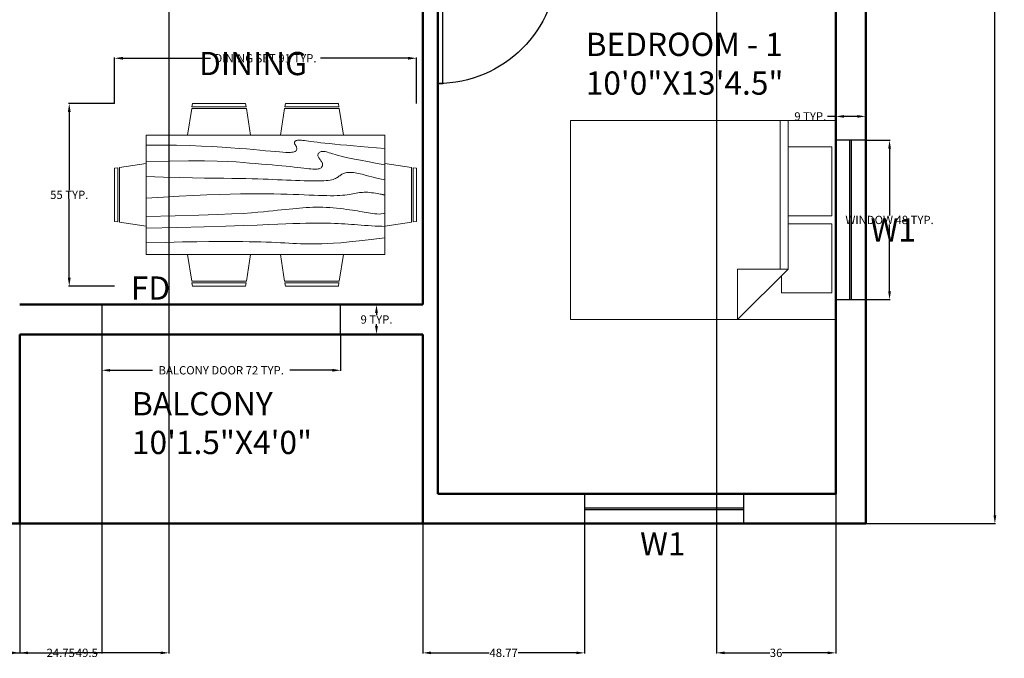
# Model space of a CAD drawing. Units: inches. Extents: x 227 to 711, y 218 to 1048.
# Tile 2 of 5: x 414 to 711, y 218 to 411. Entities that reach past the tile are written whole.
import ezdxf

# ---------------------------------------------------------------- set-up
doc = ezdxf.new("R2010")
doc.units = ezdxf.units.IN
doc.header["$MEASUREMENT"] = 0
for name, color, linetype, lineweight in [('A-ANNO-DIMS', 2, 'Continuous', 18), ('A-ANNO-TEXT', 70, 'Continuous', 18), ('A-AREA-IDEN', 70, 'Continuous', 25), ('A-FURN', 8, 'Continuous', 18), ('A-WALL', 10, 'Continuous', 50), ('DOORS', 30, 'Continuous', 25), ('WINDOWS', 50, 'Continuous', 25)]:
    doc.layers.add(name, color=color, linetype=linetype, lineweight=lineweight)
doc.styles.get("Standard").update_dxf_attribs({"font": 'arial.ttf'})
doc.dimstyles.get("Standard").update_dxf_attribs({"dimtxt": 2.5, "dimasz": 2.5, "dimexe": 0.18, "dimexo": 0.0625, "dimgap": 0.09, "dimtad": 0, "dimtih": 1, "dimtoh": 1, "dimzin": 0, "dimdsep": 46, "dimlunit": 3, "dimtxsty": 'Standard', "dimcen": 0.09, "dimadec": 0, "dimazin": 0, "dimtfac": 1, "dimtofl": 0, "dimtmove": 0, "dimatfit": 3, "dimfxl": 1, "dimtolj": 1, "dimtzin": 0, "dimarcsym": 0})

# ---------------------------------------------------------------- blocks, each defined once
blk = doc.blocks.new('*U2')
for p, q in [((0, 0), (0, -6)), ((40, 0), (40, -6))]:
    blk.add_line(p, q)
blk.add_lwpolyline([(0, 0), (0, 40), (1.75, 40), (1.75, 0)], close=True)
blk.add_arc((0, 0), 40, 0, 90)
blk = doc.blocks.new('Bed - Queen')
for p, q in [((0, -80.00003), (0, 0)), ((0, 0), (59.99999, 0)), ((59.99999, 0), (59.99999, -80.00003)), ((7.99999, -1.2), (28.79998, -1.2)), ((7.99999, -14.4), (7.99999, -1.2)), ((28.79998, -1.2), (28.79998, -14.4)), ((31.19999, -1.2), (51.99999, -1.2)), ((31.19999, -14.4), (31.19999, -1.2)), ((51.99999, -1.2), (51.99999, -16.4)), ((0, -14.4), (44.8, -14.4)), ((59.99999, -29.6), (44.8, -14.4)), ((44.8, -14.4), (44.8, -29.6)), ((44.8, -16.8), (0, -16.8)), ((51.99999, -16.4), (46.79936, -16.4)), ((44.8, -29.6), (59.99999, -29.6)), ((59.99999, -80.00003), (0, -80.00003))]:
    blk.add_line(p, q)
blk = doc.blocks.new('Dining Set - 36 x 72 in.')
for p, q in [((-22, 27.5), (-22.1562, 26.50042)), ((-22, 27.5), (-6, 27.5)), ((-5.8437, 26.49966), (-6, 27.5)), ((6, 27.5), (5.8438, 26.50042)), ((6, 27.5), (22, 27.5)), ((22.1563, 26.49966), (22, 27.5)), ((-22.2343, 26.00059), (-23.4847, 17.99762)), ((-22.2304, 26), (-5.7608, 26)), ((-5.8416, 26.5), (-22.1534, 26.5)), ((-4.5152, 17.99762), (-5.7655, 25.99926)), ((5.7657, 26.00059), (4.5153, 17.99762)), ((5.7696, 26), (22.2392, 26)), ((22.1584, 26.5), (5.8466, 26.5)), ((23.4848, 17.99762), (22.2345, 25.99926)), ((36, 18), (-36, 18)), ((-36, 18), (-36, -18)), ((36, -18), (36, 18)), ((-44.0006, 8.23428), (-35.9976, 9.48474)), ((44.0006, 8.23428), (35.9976, 9.48474)), ((-45.5, 8), (-44.5004, 8.15617)), ((-45.5, 8), (-45.5, -8)), ((-44.5, -8.15843), (-44.5, 8.15338)), ((-44, 8.23041), (-44, -8.23915)), ((44, 8.23041), (44, -8.23915)), ((44.5, -8.15843), (44.5, 8.15338)), ((45.5, 8), (44.5005, 8.15617)), ((45.5, 8), (45.5, -8)), ((-44.4997, -8.15631), (-45.5, -8)), ((-35.9976, -9.48476), (-43.9993, -8.2345)), ((35.9976, -9.48476), (43.9993, -8.2345)), ((44.4997, -8.15631), (45.5, -8)), ((-36, -18), (36, -18)), ((-22.2343, -26.0006), (-23.4847, -17.99762)), ((-4.5152, -17.99762), (-5.7655, -25.99928)), ((5.7657, -26.0006), (4.5153, -17.99762)), ((23.4848, -17.99762), (22.2345, -25.99928)), ((-22.2304, -26), (-5.7608, -26)), ((-22, -27.5), (-22.1562, -26.50044)), ((-5.8416, -26.5), (-22.1534, -26.5)), ((-5.8437, -26.49967), (-6, -27.5)), ((5.7696, -26), (22.2392, -26)), ((6, -27.5), (5.8438, -26.50044)), ((22.1584, -26.5), (5.8466, -26.5)), ((22.1563, -26.49967), (22, -27.5)), ((-22, -27.5), (-6, -27.5)), ((6, -27.5), (22, -27.5))]:
    blk.add_line(p, q)
for points in [[(-36, 15), (-31.1772, 14.97754), (-26.8079, 14.91406), (-22.8538, 14.81543), (-19.276, 14.6875), (-16.0362, 14.53613), (-13.0957, 14.36718), (-10.4159, 14.18652), (-7.9583, 14), (-5.6904, 13.81315), (-3.6035, 13.63021), (-1.6954, 13.45508), (0.0365, 13.29166), (1.5945, 13.14388), (2.9811, 13.01562), (4.1988, 12.9108), (5.25, 12.83333), (6.1393, 12.78613), (6.8802, 12.76823), (7.4883, 12.77767), (7.9792, 12.8125), (8.3685, 12.87077), (8.6719, 12.95052), (8.9049, 13.0498), (9.0833, 13.16666), (9.2205, 13.29899), (9.3216, 13.44401), (9.3895, 13.59879), (9.4271, 13.76041), (9.4373, 13.92594), (9.4232, 14.09245), (9.3875, 14.257), (9.3333, 14.41666), (9.2638, 14.56917), (9.1836, 14.71484), (9.0975, 14.85465), (9.0104, 14.98958), (8.9272, 15.1206), (8.8529, 15.2487), (8.7922, 15.37483), (8.75, 15.5), (8.7305, 15.62467), (8.7344, 15.74739), (8.7617, 15.86621), (8.8125, 15.97916), (8.8867, 16.08431), (8.9844, 16.17968), (9.1055, 16.26334), (9.25, 16.33333), (9.4189, 16.38802), (9.6172, 16.42708), (9.8506, 16.45052), (10.125, 16.45833), (10.4463, 16.45052), (10.8203, 16.42708), (11.2529, 16.38802), (11.75, 16.33333), (12.3184, 16.26318), (12.9694, 16.17838), (13.7151, 16.07991), (14.5677, 15.96875), (15.5395, 15.84586), (16.6426, 15.71224), (17.8893, 15.56884), (19.2917, 15.41666), (20.859, 15.25667), (22.5879, 15.08984), (24.4721, 14.91715), (26.5052, 14.73958), (28.6809, 14.5581), (30.9929, 14.3737), (33.4347, 14.18733), (36, 14)], [(-36, 10), (-28.9766, 10.14274), (-23.1725, 10.20442), (-18.4241, 10.19775), (-14.5677, 10.13541), (-11.4399, 10.03011), (-8.877, 9.89453), (-6.7154, 9.74137), (-4.7917, 9.58333), (-2.9698, 9.43082), (-1.2246, 9.28515), (0.4415, 9.14534), (2.026, 9.01041), (3.5266, 8.87939), (4.9408, 8.7513), (6.266, 8.62516), (7.5, 8.5), (8.6411, 8.37549), (9.6914, 8.2539), (10.6538, 8.13818), (11.5312, 8.03125), (12.3267, 7.93603), (13.043, 7.85547), (13.6831, 7.79248), (14.25, 7.75), (14.7471, 7.7303), (15.1797, 7.73307), (15.5537, 7.75732), (15.875, 7.80208), (16.1494, 7.86637), (16.3828, 7.94922), (16.5811, 8.04964), (16.75, 8.16666), (16.8944, 8.29915), (17.0143, 8.44531), (17.1089, 8.60319), (17.1771, 8.77083), (17.218, 8.94629), (17.2305, 9.1276), (17.2137, 9.31282), (17.1667, 9.5), (17.0895, 9.6875), (16.987, 9.875), (16.8649, 10.0625), (16.7292, 10.25), (16.5856, 10.4375), (16.4401, 10.625), (16.2985, 10.8125), (16.1667, 11), (16.05, 11.18733), (15.9518, 11.3737), (15.8752, 11.5581), (15.8229, 11.73958), (15.798, 11.91715), (15.8034, 12.08984), (15.842, 12.25667), (15.9167, 12.41666), (16.0295, 12.56836), (16.1784, 12.70833), (16.3605, 12.83268), (16.5729, 12.9375), (16.8127, 13.01888), (17.0768, 13.07291), (17.3625, 13.0957), (17.6667, 13.08333), (17.9894, 13.03312), (18.3418, 12.94726), (18.7382, 12.82918), (19.1927, 12.68229), (19.7195, 12.51001), (20.3327, 12.31575), (21.0465, 12.10294), (21.875, 11.875), (22.8357, 11.63354), (23.959, 11.37304), (25.2786, 11.08618), (26.8282, 10.76562), (28.6414, 10.40405), (30.752, 9.99414), (33.1936, 9.52856), (36, 9)], [(-36, 5.5), (-30.7157, 5.3348), (-26.069, 5.20963), (-21.9946, 5.11767), (-18.4271, 5.05208), (-15.3009, 5.00602), (-12.5508, 4.97265), (-10.1112, 4.94515), (-7.9167, 4.91666), (-5.909, 4.88167), (-4.0586, 4.83984), (-2.3429, 4.79215), (-0.7396, 4.73958), (0.7739, 4.6831), (2.22, 4.6237), (3.6213, 4.56233), (5, 4.5), (6.373, 4.43782), (7.7344, 4.3776), (9.0723, 4.32129), (10.375, 4.27083), (11.6309, 4.22819), (12.8281, 4.19531), (13.9551, 4.17415), (15, 4.16666), (15.954, 4.17448), (16.819, 4.19791), (17.6001, 4.23698), (18.3021, 4.29166), (18.9299, 4.36198), (19.4883, 4.44791), (19.9823, 4.54948), (20.4167, 4.66666), (20.7969, 4.79899), (21.1302, 4.94401), (21.4245, 5.09879), (21.6875, 5.26041), (21.9271, 5.42594), (22.1511, 5.59245), (22.3672, 5.757), (22.5834, 5.91666), (22.8065, 6.06868), (23.0404, 6.21093), (23.2879, 6.34147), (23.5521, 6.45833), (23.8358, 6.55957), (24.142, 6.64323), (24.4735, 6.70735), (24.8334, 6.75), (25.2235, 6.76969), (25.642, 6.76692), (26.0858, 6.74267), (26.5521, 6.69791), (27.0379, 6.63362), (27.5404, 6.55078), (28.0565, 6.45036), (28.5834, 6.33333), (29.1242, 6.19987), (29.7071, 6.04687), (30.3661, 5.87044), (31.1354, 5.66666), (32.0493, 5.43164), (33.142, 5.16146), (34.4475, 4.85221), (36, 4.5)], [(-36, -1), (-30.7915, -0.6591), (-26.0195, -0.38216), (-21.6519, -0.16284), (-17.6563, 0.00521), (-14.0005, 0.12833), (-10.6523, 0.21289), (-7.5796, 0.26522), (-4.75, 0.29166), (-2.134, 0.29793), (0.2878, 0.28711), (2.5317, 0.26163), (4.6146, 0.22396), (6.5529, 0.17651), (8.3633, 0.12174), (10.0623, 0.06209), (11.6667, 0), (13.1899, -0.06201), (14.6341, -0.1211), (15.9982, -0.17432), (17.2813, -0.21875), (18.4823, -0.25147), (19.6003, -0.26953), (20.6343, -0.27002), (21.5834, -0.25), (22.4481, -0.20768), (23.2357, -0.14584), (23.9549, -0.06836), (24.6146, 0.02083), (25.2235, 0.11784), (25.7904, 0.21875), (26.3241, 0.31966), (26.8334, 0.41666), (27.3265, 0.50618), (27.8099, 0.58593), (28.2894, 0.65397), (28.7709, 0.70833), (29.2601, 0.74707), (29.763, 0.76823), (30.2855, 0.76985), (30.8334, 0.75), (31.4088, 0.70784), (31.9994, 0.64713), (32.589, 0.57275), (33.1615, 0.48958), (33.7008, 0.4025), (34.1908, 0.3164), (34.6153, 0.23616), (34.9584, 0.16666), (35.2099, 0.11165), (35.3848, 0.07031), (35.504, 0.04069), (35.5886, 0.02083), (35.6594, 0.00879), (35.7377, 0.0026), (35.8442, 0.00032), (36, 0)], [(-36, -6.5), (-27.1843, -6.31267), (-20.084, -6.1263), (-14.469, -5.9419), (-10.1094, -5.76042), (-6.7752, -5.58285), (-4.2363, -5.41016), (-2.2629, -5.24333), (-0.625, -5.08334), (0.8708, -4.93099), (2.2715, -4.78646), (3.5872, -4.64974), (4.8281, -4.52084), (6.0046, -4.39974), (7.127, -4.28646), (8.2053, -4.18099), (9.25, -4.08334), (10.2705, -3.99382), (11.2734, -3.91407), (12.2647, -3.84603), (13.25, -3.79167), (14.2354, -3.75293), (15.2266, -3.73177), (16.2295, -3.73015), (17.25, -3.75), (18.2912, -3.79248), (19.3451, -3.85547), (20.4009, -3.93604), (21.4479, -4.03125), (22.4754, -4.13819), (23.4727, -4.25391), (24.4289, -4.37549), (25.3334, -4.5), (26.1785, -4.62492), (26.9694, -4.74935), (27.7145, -4.87281), (28.4219, -4.99479), (29.1, -5.11483), (29.7572, -5.23242), (30.4016, -5.34709), (31.0417, -5.45834), (31.6837, -5.56437), (32.3262, -5.65821), (32.9658, -5.73153), (33.599, -5.77604), (34.2224, -5.78345), (34.8327, -5.74545), (35.4264, -5.65373), (36, -5.5)], [(-36, -10), (-26.4022, -9.81299), (-18.4675, -9.62891), (-11.9839, -9.45069), (-6.7396, -9.28125), (-2.5226, -9.12354), (0.8789, -8.98047), (3.6769, -8.85498), (6.0833, -8.75), (8.2767, -8.66765), (10.3021, -8.60677), (12.1712, -8.56543), (13.8958, -8.54167), (15.4876, -8.53353), (16.9583, -8.53907), (18.3197, -8.55632), (19.5834, -8.58334), (20.7616, -8.61841), (21.8685, -8.66081), (22.9188, -8.71004), (23.9271, -8.76563), (24.9081, -8.82707), (25.8763, -8.89388), (26.8465, -8.96558), (27.8334, -9.04167), (28.8474, -9.12118), (29.8828, -9.20117), (30.93, -9.27824), (31.9792, -9.34896), (33.0205, -9.40991), (34.0443, -9.45768), (35.0407, -9.48885), (36, -9.5)], [(-36, -14.5), (-30.0881, -14.33513), (-25.0332, -14.21224), (-20.7312, -14.12647), (-17.0781, -14.07292), (-13.97, -14.04671), (-11.3027, -14.04297), (-8.9724, -14.05681), (-6.875, -14.08334), (-4.9224, -14.11833), (-3.0905, -14.16016), (-1.3709, -14.20785), (0.2448, -14.26042), (1.7647, -14.3169), (3.1973, -14.3763), (4.5507, -14.43767), (5.8333, -14.5), (7.0554, -14.5621), (8.235, -14.62175), (9.3922, -14.67652), (10.5469, -14.72396), (11.7192, -14.76164), (12.929, -14.78711), (14.1965, -14.79794), (15.5417, -14.79167), (16.9933, -14.76424), (18.6152, -14.70508), (20.4804, -14.60197), (22.6615, -14.44271), (25.2312, -14.21509), (28.2624, -13.9069), (31.8277, -13.50594), (36, -13)]]:
    blk.add_lwpolyline(points)
blk = doc.blocks.new('WIN-48IN')
for p, q in [((0, 4.75), (48, 4.75)), ((0, 4.25), (48, 4.25))]:
    blk.add_line(p, q)
blk.add_lwpolyline([(0, 0), (48, 0), (48, 9), (0, 9)], close=True)
blk = doc.blocks.new('DOOR-FD-72IN')
blk.add_lwpolyline([(0, 0), (72, 0), (72, 9), (0, 9)], close=True)
blk = doc.blocks.new('*D20')
at = {"layer": 'A-ANNO-DIMS', "color": 0, "lineweight": -2, "transparency": 16777216}
for p, q in [((669.55, 374.57), (676.87, 374.57)), ((676.69, 372.07), (676.69, 351.95)), ((676.69, 329.07), (676.69, 349.18)), ((669.55, 326.57), (676.87, 326.57))]:
    blk.add_line(p, q, dxfattribs=at)
at = {"layer": 'A-ANNO-DIMS', "color": 0, "transparency": 16777216}
for points in [[(676.27, 372.07), (677.11, 372.07), (676.69, 374.57)], [(676.27, 329.07), (677.11, 329.07), (676.69, 326.57)]]:
    blk.add_solid(points, dxfattribs=at)
at = {"layer": 'Defpoints', "color": 0, "transparency": 16777216}
for p in [(669.49, 374.57), (676.69, 374.57), (669.49, 326.57)]:
    blk.add_point(p, dxfattribs=at)
at = {"layer": 'A-ANNO-DIMS', "color": 0, "transparency": 16777216, "insert": (676.69, 350.57), "char_height": 2.5, "attachment_point": 5}
blk.add_mtext('\\A1;WINDOW 48 TYP.', dxfattribs=at)
blk = doc.blocks.new('*D21')
at = {"layer": 'A-ANNO-DIMS', "color": 0, "lineweight": -2, "transparency": 16777216}
for p, q in [((660.49, 381.77), (657.99, 381.77)), ((660.49, 374.63), (660.49, 381.95)), ((666.99, 381.77), (662.99, 381.77)), ((669.49, 374.63), (669.49, 381.95))]:
    blk.add_line(p, q, dxfattribs=at)
at = {"layer": 'A-ANNO-DIMS', "color": 0, "transparency": 16777216}
for points in [[(662.99, 382.18), (662.99, 381.35), (660.49, 381.77)], [(666.99, 382.18), (666.99, 381.35), (669.49, 381.77)]]:
    blk.add_solid(points, dxfattribs=at)
at = {"layer": 'Defpoints', "color": 0, "transparency": 16777216}
for p in [(660.49, 381.77), (660.49, 374.57), (669.49, 374.57)]:
    blk.add_point(p, dxfattribs=at)
at = {"layer": 'A-ANNO-DIMS', "color": 0, "transparency": 16777216, "insert": (652.79, 381.77), "char_height": 2.5, "attachment_point": 5}
blk.add_mtext('\\A1;9 TYP.', dxfattribs=at)
blk = doc.blocks.new('*D36')
at = {"layer": 'A-ANNO-DIMS', "color": 0, "lineweight": -2, "transparency": 16777216}
for p, q in [((443.08, 385.7), (443.08, 399.47)), ((445.58, 399.29), (471.99, 399.29)), ((531.58, 399.29), (505.17, 399.29)), ((534.08, 385.7), (534.08, 399.47))]:
    blk.add_line(p, q, dxfattribs=at)
at = {"layer": 'A-ANNO-DIMS', "color": 0, "transparency": 16777216}
for points in [[(445.58, 399.71), (445.58, 398.87), (443.08, 399.29)], [(531.58, 399.71), (531.58, 398.87), (534.08, 399.29)]]:
    blk.add_solid(points, dxfattribs=at)
at = {"layer": 'Defpoints', "color": 0, "transparency": 16777216}
for p in [(534.08, 399.29), (443.08, 385.64), (534.08, 385.64)]:
    blk.add_point(p, dxfattribs=at)
at = {"layer": 'A-ANNO-DIMS', "color": 0, "transparency": 16777216, "insert": (488.58, 399.29), "char_height": 2.5, "attachment_point": 5}
blk.add_mtext('\\A1;DINING SET 91 TYP.', dxfattribs=at)
blk = doc.blocks.new('*D37')
at = {"layer": 'A-ANNO-DIMS', "color": 0, "lineweight": -2, "transparency": 16777216}
for p, q in [((443.02, 385.64), (429.25, 385.64)), ((429.43, 383.14), (429.43, 359.5)), ((429.43, 333.14), (429.43, 356.78)), ((443.02, 330.64), (429.25, 330.64))]:
    blk.add_line(p, q, dxfattribs=at)
at = {"layer": 'A-ANNO-DIMS', "color": 0, "transparency": 16777216}
for points in [[(429.01, 383.14), (429.85, 383.14), (429.43, 385.64)], [(429.01, 333.14), (429.85, 333.14), (429.43, 330.64)]]:
    blk.add_solid(points, dxfattribs=at)
at = {"layer": 'Defpoints', "color": 0, "transparency": 16777216}
for p in [(429.43, 385.64), (443.08, 385.64), (443.08, 330.64)]:
    blk.add_point(p, dxfattribs=at)
at = {"layer": 'A-ANNO-DIMS', "color": 0, "transparency": 16777216, "insert": (429.43, 358.14), "char_height": 2.5, "attachment_point": 5}
blk.add_mtext('\\A1;55 TYP.', dxfattribs=at)
blk = doc.blocks.new('*D40')
at = {"layer": 'A-ANNO-DIMS', "color": 0, "lineweight": -2, "transparency": 16777216}
for p, q in [((439.24, 316), (439.24, 305.09)), ((511.24, 316), (511.24, 305.09)), ((441.74, 305.27), (454.57, 305.27)), ((508.74, 305.27), (495.91, 305.27))]:
    blk.add_line(p, q, dxfattribs=at)
at = {"layer": 'A-ANNO-DIMS', "color": 0, "transparency": 16777216}
for points in [[(441.74, 305.68), (441.74, 304.85), (439.24, 305.27)], [(508.74, 305.68), (508.74, 304.85), (511.24, 305.27)]]:
    blk.add_solid(points, dxfattribs=at)
at = {"layer": 'Defpoints', "color": 0, "transparency": 16777216}
for p in [(439.24, 316.07), (511.24, 316.07), (511.24, 305.27)]:
    blk.add_point(p, dxfattribs=at)
at = {"layer": 'A-ANNO-DIMS', "color": 0, "transparency": 16777216, "insert": (475.24, 305.27), "char_height": 2.5, "attachment_point": 5}
blk.add_mtext('\\A1;BALCONY DOOR 72 TYP.', dxfattribs=at)
blk = doc.blocks.new('*D41')
at = {"layer": 'A-ANNO-DIMS', "color": 0, "lineweight": -2, "transparency": 16777216}
for p, q in [((511.3, 325.07), (522.22, 325.07)), ((522.04, 322.57), (522.04, 321.93)), ((522.04, 318.57), (522.04, 319.2)), ((511.3, 316.07), (522.22, 316.07))]:
    blk.add_line(p, q, dxfattribs=at)
at = {"layer": 'A-ANNO-DIMS', "color": 0, "transparency": 16777216}
for points in [[(521.62, 322.57), (522.46, 322.57), (522.04, 325.07)], [(521.62, 318.57), (522.46, 318.57), (522.04, 316.07)]]:
    blk.add_solid(points, dxfattribs=at)
at = {"layer": 'Defpoints', "color": 0, "transparency": 16777216}
for p in [(511.24, 325.07), (522.04, 325.07), (511.24, 316.07)]:
    blk.add_point(p, dxfattribs=at)
at = {"layer": 'A-ANNO-DIMS', "color": 0, "transparency": 16777216, "insert": (522.04, 320.57), "char_height": 2.5, "attachment_point": 5}
blk.add_mtext('\\A1;9 TYP.', dxfattribs=at)
blk = doc.blocks.new('*D45')
at = {"layer": 'A-ANNO-DIMS', "color": 0, "lineweight": -2, "transparency": 16777216}
for p, q in [((669.55, 1007.07), (708.62, 1007.07)), ((708.44, 1004.57), (708.44, 634.43)), ((708.44, 261.57), (708.44, 631.7)), ((669.55, 259.07), (708.62, 259.07))]:
    blk.add_line(p, q, dxfattribs=at)
at = {"layer": 'A-ANNO-DIMS', "color": 0, "transparency": 16777216}
for points in [[(708.02, 1004.57), (708.86, 1004.57), (708.44, 1007.07)], [(708.02, 261.57), (708.86, 261.57), (708.44, 259.07)]]:
    blk.add_solid(points, dxfattribs=at)
at = {"layer": 'Defpoints', "color": 0, "transparency": 16777216}
for p in [(669.49, 1007.07), (708.44, 1007.07), (669.49, 259.07)]:
    blk.add_point(p, dxfattribs=at)
at = {"layer": 'A-ANNO-DIMS', "color": 0, "transparency": 16777216, "insert": (708.44, 633.07), "char_height": 2.5, "attachment_point": 5}
blk.add_mtext('\\A1;748', dxfattribs=at)
blk = doc.blocks.new('*D48')
at = {"layer": 'A-ANNO-DIMS', "color": 0, "lineweight": -2, "transparency": 16777216}
for p, q in [((385.24, 259), (385.24, 219.94)), ((414.49, 259), (414.49, 219.94)), ((387.74, 220.12), (395.53, 220.12)), ((411.99, 220.12), (404.2, 220.12))]:
    blk.add_line(p, q, dxfattribs=at)
at = {"layer": 'A-ANNO-DIMS', "color": 0, "transparency": 16777216}
for points in [[(387.74, 220.53), (387.74, 219.7), (385.24, 220.12)], [(411.99, 220.53), (411.99, 219.7), (414.49, 220.12)]]:
    blk.add_solid(points, dxfattribs=at)
at = {"layer": 'Defpoints', "color": 0, "transparency": 16777216}
for p in [(385.24, 259.07), (414.49, 259.07), (414.49, 220.12)]:
    blk.add_point(p, dxfattribs=at)
at = {"layer": 'A-ANNO-DIMS', "color": 0, "transparency": 16777216, "insert": (399.86, 220.12), "char_height": 2.5, "attachment_point": 5}
blk.add_mtext('\\A1;29.25', dxfattribs=at)
blk = doc.blocks.new('*D49')
at = {"layer": 'A-ANNO-DIMS', "color": 0, "lineweight": -2, "transparency": 16777216}
for p, q in [((535.99, 259), (535.99, 219.94)), ((584.76, 259), (584.76, 219.94)), ((538.49, 220.12), (556.01, 220.12)), ((582.26, 220.12), (564.73, 220.12))]:
    blk.add_line(p, q, dxfattribs=at)
at = {"layer": 'A-ANNO-DIMS', "color": 0, "transparency": 16777216}
for points in [[(538.49, 220.53), (538.49, 219.7), (535.99, 220.12)], [(582.26, 220.53), (582.26, 219.7), (584.76, 220.12)]]:
    blk.add_solid(points, dxfattribs=at)
at = {"layer": 'Defpoints', "color": 0, "transparency": 16777216}
for p in [(535.99, 259.07), (584.76, 259.07), (584.76, 220.12)]:
    blk.add_point(p, dxfattribs=at)
at = {"layer": 'A-ANNO-DIMS', "color": 0, "transparency": 16777216, "insert": (560.37, 220.12), "char_height": 2.5, "attachment_point": 5}
blk.add_mtext('\\A1;48.77', dxfattribs=at)
blk = doc.blocks.new('*D60')
at = {"layer": 'A-ANNO-DIMS', "color": 0, "lineweight": -2, "transparency": 16777216}
for p, q in [((459.49, 681), (459.49, 219.94)), ((409.99, 636), (409.99, 219.94)), ((412.49, 220.12), (431.34, 220.12)), ((456.99, 220.12), (438.14, 220.12))]:
    blk.add_line(p, q, dxfattribs=at)
at = {"layer": 'A-ANNO-DIMS', "color": 0, "transparency": 16777216}
for points in [[(412.49, 220.53), (412.49, 219.7), (409.99, 220.12)], [(456.99, 220.53), (456.99, 219.7), (459.49, 220.12)]]:
    blk.add_solid(points, dxfattribs=at)
at = {"layer": 'Defpoints', "color": 0, "transparency": 16777216}
for p in [(459.49, 681.07), (409.99, 636.07), (459.49, 220.12)]:
    blk.add_point(p, dxfattribs=at)
at = {"layer": 'A-ANNO-DIMS', "color": 0, "transparency": 16777216, "insert": (434.74, 220.12), "char_height": 2.5, "attachment_point": 5}
blk.add_mtext('\\A1;49.5', dxfattribs=at)
blk = doc.blocks.new('*D62')
at = {"layer": 'A-ANNO-DIMS', "color": 0, "lineweight": -2, "transparency": 16777216}
for p, q in [((624.49, 998), (624.49, 219.94)), ((660.49, 998), (660.49, 219.94)), ((626.99, 220.12), (640.61, 220.12)), ((657.99, 220.12), (644.37, 220.12))]:
    blk.add_line(p, q, dxfattribs=at)
at = {"layer": 'A-ANNO-DIMS', "color": 0, "transparency": 16777216}
for points in [[(626.99, 220.53), (626.99, 219.7), (624.49, 220.12)], [(657.99, 220.53), (657.99, 219.7), (660.49, 220.12)]]:
    blk.add_solid(points, dxfattribs=at)
at = {"layer": 'Defpoints', "color": 0, "transparency": 16777216}
for p in [(624.49, 998.07), (660.49, 998.07), (660.49, 220.12)]:
    blk.add_point(p, dxfattribs=at)
at = {"layer": 'A-ANNO-DIMS', "color": 0, "transparency": 16777216, "insert": (642.49, 220.12), "char_height": 2.5, "attachment_point": 5}
blk.add_mtext('\\A1;36', dxfattribs=at)
blk = doc.blocks.new('*D64')
at = {"layer": 'A-ANNO-DIMS', "color": 0, "lineweight": -2, "transparency": 16777216}
for p, q in [((414.49, 316), (414.49, 219.94)), ((439.24, 316), (439.24, 219.94)), ((416.99, 220.12), (422.53, 220.12)), ((436.74, 220.12), (431.2, 220.12))]:
    blk.add_line(p, q, dxfattribs=at)
at = {"layer": 'A-ANNO-DIMS', "color": 0, "transparency": 16777216}
for points in [[(416.99, 220.53), (416.99, 219.7), (414.49, 220.12)], [(436.74, 220.53), (436.74, 219.7), (439.24, 220.12)]]:
    blk.add_solid(points, dxfattribs=at)
at = {"layer": 'Defpoints', "color": 0, "transparency": 16777216}
for p in [(414.49, 316.07), (439.24, 316.07), (439.24, 220.12)]:
    blk.add_point(p, dxfattribs=at)
at = {"layer": 'A-ANNO-DIMS', "color": 0, "transparency": 16777216, "insert": (426.86, 220.12), "char_height": 2.5, "attachment_point": 5}
blk.add_mtext('\\A1;24.75', dxfattribs=at)

msp = doc.modelspace()

# ---------------------------------------------------------------- linework, layer by layer
at = {"layer": 'A-WALL'}
for p, q in [((535.99, 433.065), (535.99, 325.065)), ((540.49, 433.065), (540.49, 268.065)), ((660.49, 268.065), (660.49, 433.065)), ((414.49, 325.065), (535.99, 325.065)), ((414.49, 316.065), (535.99, 316.065)), ((414.49, 316.065), (414.49, 259.065)), ((535.99, 316.065), (535.99, 259.065)), ((540.49, 268.065), (660.49, 268.065)), ((414.49, 259.065), (535.99, 259.065))]:
    msp.add_line(p, q, dxfattribs=at)
for points in [[(414.49, 1007.065), (268.99, 1007.065), (268.99, 259.065), (414.49, 259.065)], [(535.99, 259.065), (669.49, 259.065), (669.49, 1007.065), (535.99, 1007.065)]]:
    msp.add_lwpolyline(points, dxfattribs=at)

# ---------------------------------------------------------------- block references
at = {"layer": 'A-FURN'}
msp.add_blockref('Dining Set - 36 x 72 in.', (488.581, 358.139), dxfattribs=at)
at = {"layer": 'A-FURN', "rotation": 270}
msp.add_blockref('Bed - Queen', (660.49, 380.565), dxfattribs=at)
at = {"layer": 'DOORS', "xscale": -0.9000000000000039, "yscale": 0.9000000000000039, "zscale": 0.9000000000000039, "rotation": 180}
msp.add_blockref('*U2', (540.49, 427.665), dxfattribs=at)
at = {"layer": 'DOORS'}
msp.add_blockref('DOOR-FD-72IN', (439.24, 316.065), dxfattribs=at)
at = {"layer": 'WINDOWS', "rotation": 89.99999999999976}
msp.add_blockref('WIN-48IN', (669.49, 326.565), dxfattribs=at)
at = {"layer": 'WINDOWS'}
msp.add_blockref('WIN-48IN', (584.755, 259.065), dxfattribs=at)

# ---------------------------------------------------------------- texts
at = {"layer": 'A-ANNO-TEXT', "char_height": 7, "attachment_point": 1}
for s, insert in [('W1', (670.95, 351.059)), ('FD', (448.008, 333.54)), ('W1', (601.496, 256.458))]:
    msp.add_mtext_dynamic_manual_height_columns(s, width=74.58955, gutter_width=1, heights=[0], dxfattribs=dict(at, insert=insert))
at = {"layer": 'A-AREA-IDEN', "char_height": 7, "attachment_point": 1}
for s, insert in [('BEDROOM - 1\\P10\'0"X13\'4.5"', (585.114, 406.983)), ('DINING', (468.55, 401.196)), ('BALCONY\\P10\'1.5"X4\'0"', (448.328, 298.689))]:
    msp.add_mtext_dynamic_manual_height_columns(s, width=74.58955, gutter_width=1, heights=[0], dxfattribs=dict(at, insert=insert))

# ---------------------------------------------------------------- dimensions: what is measured, and where the dimension line sits
at = {"layer": 'A-ANNO-DIMS'}
dim = msp.add_linear_dim(base=(708.44, 1007.065), p1=(669.49, 259.065), p2=(669.49, 1007.065), angle=90, dimstyle='Standard', override={"dimdec": 0, "dimlfac": 1, "dimrnd": 0, "dimzin": 0, "dimdsep": 46, "dimlunit": 2}, dxfattribs=at)
dim.commit()
dim.dimension.update_dxf_attribs({"geometry": '*D45', "text_midpoint": (708.44, 633.065)})
for base, p1, p2, override, picture, middle in [((660.49, 220.115), (624.49, 998.065), (660.49, 998.065), {"dimdec": 0, "dimlfac": 1, "dimrnd": 0, "dimzin": 0, "dimdsep": 46, "dimlunit": 2}, '*D62', (642.49, 220.115)), ((459.49, 220.115), (409.99, 636.065), (459.49, 681.065), {"dimdec": 1, "dimlfac": 1, "dimrnd": 0, "dimzin": 0, "dimdsep": 46, "dimlunit": 2}, '*D60', (434.74, 220.115)), ((439.24, 220.115), (414.49, 316.065), (439.24, 316.065), {"dimdec": 2, "dimlfac": 1, "dimrnd": 0, "dimzin": 0, "dimdsep": 46, "dimlunit": 2}, '*D64', (426.865, 220.115)), ((414.49, 220.115), (385.24, 259.065), (414.49, 259.065), {"dimdec": 2, "dimlfac": 1, "dimrnd": 0, "dimzin": 0, "dimdsep": 46, "dimlunit": 2}, '*D48', (399.865, 220.115)), ((584.7553, 220.115), (535.9899, 259.065), (584.7553, 259.065), {"dimdec": 2, "dimlfac": 1, "dimrnd": 0, "dimzin": 0, "dimdsep": 46, "dimlunit": 2}, '*D49', (560.3726, 220.115))]:
    dim = msp.add_linear_dim(base=base, p1=p1, p2=p2, dimstyle='Standard', override=override, dxfattribs=at)
    dim.commit()
    dim.dimension.update_dxf_attribs({"geometry": picture, "text_midpoint": middle})
for base, p1, p2, text, picture, middle in [((534.081, 399.289), (443.081, 385.639), (534.081, 385.639), 'DINING SET <> TYP.', '*D36', (488.581, 399.289)), ((511.24, 305.265), (439.24, 316.065), (511.24, 316.065), 'BALCONY DOOR <> TYP.', '*D40', (475.24, 305.265))]:
    dim = msp.add_linear_dim(base=base, p1=p1, p2=p2, text=text, dimstyle='Standard', override={"dimdec": 0, "dimlfac": 1, "dimrnd": 0, "dimzin": 0, "dimdsep": 46, "dimlunit": 2}, dxfattribs=at)
    dim.commit()
    dim.dimension.update_dxf_attribs({"geometry": picture, "text_midpoint": middle})
for base, p1, p2, angle, text, picture, middle in [((429.431, 385.639), (443.081, 330.639), (443.081, 385.639), 90, '<> TYP.', '*D37', (429.431, 358.139)), ((660.49, 381.765), (669.49, 374.565), (660.49, 374.565), 180, '<> TYP.', '*D21', (652.787, 381.765)), ((676.69, 374.565), (669.49, 326.565), (669.49, 374.565), 90, 'WINDOW <> TYP.', '*D20', (676.69, 350.565)), ((522.04, 325.065), (511.24, 316.065), (511.24, 325.065), 90, '<> TYP.', '*D41', (522.04, 320.565))]:
    dim = msp.add_linear_dim(base=base, p1=p1, p2=p2, angle=angle, text=text, dimstyle='Standard', override={"dimdec": 0, "dimlfac": 1, "dimrnd": 0, "dimzin": 0, "dimdsep": 46, "dimlunit": 2}, dxfattribs=at)
    dim.commit()
    dim.dimension.update_dxf_attribs({"geometry": picture, "text_midpoint": middle})

doc.saveas('drawing.dxf')
